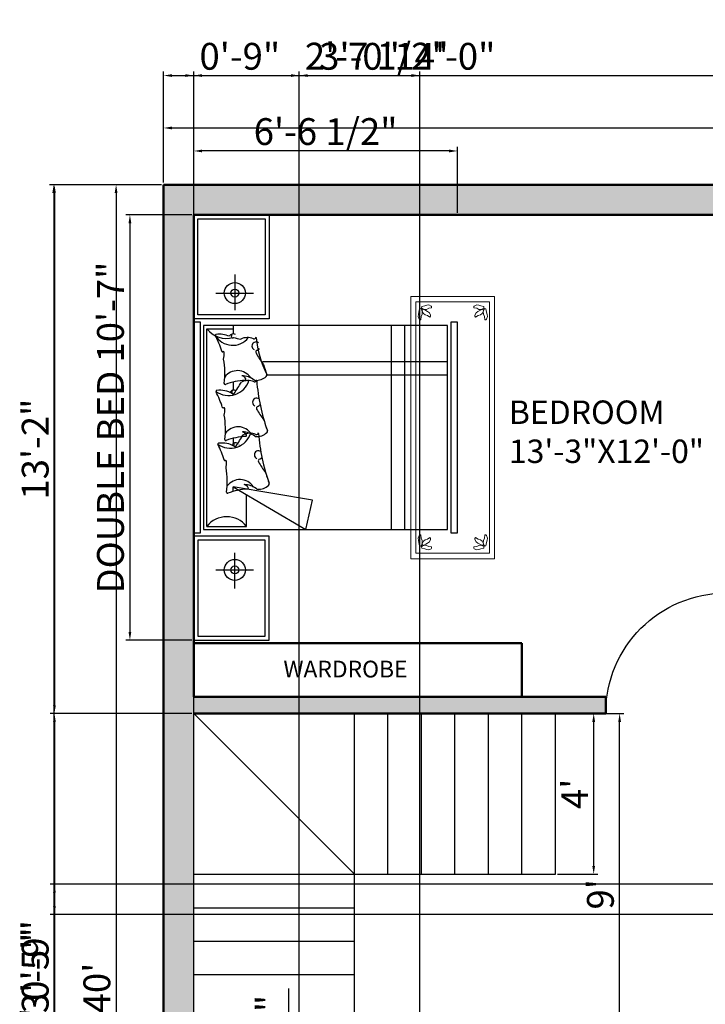
# Model space of a CAD drawing. Units: inches. Extents: x 1770 to 3141, y 984 to 1614.
# Tile 3 of 12: x 1770 to 1974, y 1320 to 1614. Entities that reach past the tile are written whole.
import ezdxf

# ---------------------------------------------------------------- set-up
doc = ezdxf.new("R2010")
doc.units = ezdxf.units.IN
for name, color, linetype, lineweight in [('A-ANNO-DIMS', 2, 'Continuous', 18), ('A-AREA-IDEN', 3, 'Continuous', 18), ('A-DOOR', 4, 'Continuous', 25), ('A-FLOR-STRS', 7, 'Continuous', 25), ('A-FURN', 8, 'Continuous', 18), ('A-WALL', 7, 'Continuous', 50), ('A-WALL-PATT', 8, 'Continuous', 13)]:
    doc.layers.add(name, color=color, linetype=linetype, lineweight=lineweight)
for name, color, linetype in [('FUR', 42, 'Continuous'), ('HA', 9, 'Continuous'), ('HID', 11, 'Continuous'), ('SAN', 5, 'Continuous')]:
    doc.layers.add(name, color=color, linetype=linetype)
doc.styles.get("Standard").update_dxf_attribs({"font": 'arial.ttf'})
doc.dimstyles.new('ISO-25', dxfattribs={"dimtxt": 8, "dimasz": 2.5, "dimexe": 1.25, "dimexo": 0.625, "dimtad": 1, "dimdec": 1, "dimlunit": 3, "dimtxsty": 'Standard', "dimcen": 2.5, "dimclrt": 1, "dimadec": 0, "dimazin": 0, "dimtfac": 1, "dimtdec": 1, "dimtmove": 0, "dimatfit": 3, "dimfxl": 1, "dimarcsym": 0})

# ---------------------------------------------------------------- blocks, each defined once
blk = doc.blocks.new("D1 3'")
for p, q in [((0, 36), (0, 0)), ((1, 36), (1, 0)), ((0, 0), (1, 0))]:
    blk.add_line(p, q)
blk.add_arc((0, 0), 36, 0, 90)
blk = doc.blocks.new('*D17')
at = {"layer": 'A-ANNO-DIMS', "color": 0, "lineweight": -2, "transparency": 16777216}
for p, q in [((1812.73, 1565.8), (1812.73, 1583.37)), ((2412.73, 1565.8), (2412.73, 1583.37)), ((1815.23, 1582.12), (2410.23, 1582.12))]:
    blk.add_line(p, q, dxfattribs=at)
at = {"layer": 'A-ANNO-DIMS', "color": 0, "transparency": 16777216}
for points in [[(1815.23, 1582.54), (1815.23, 1581.7), (1812.73, 1582.12)], [(2410.23, 1582.54), (2410.23, 1581.7), (2412.73, 1582.12)]]:
    blk.add_solid(points, dxfattribs=at)
at = {"layer": 'Defpoints', "color": 0, "transparency": 16777216}
for p in [(2412.73, 1582.12), (1812.73, 1565.18), (2412.73, 1565.18)]:
    blk.add_point(p, dxfattribs=at)
at = {"layer": 'A-ANNO-DIMS', "color": 0, "transparency": 16777216, "insert": (2112.73, 1586.83), "char_height": 8, "attachment_point": 5}
blk.add_mtext("50'", dxfattribs=at)
blk = doc.blocks.new('*D18')
at = {"layer": 'A-ANNO-DIMS', "color": 0, "lineweight": -2, "transparency": 16777216}
for p, q in [((1812.11, 1565.18), (1797.29, 1565.18)), ((1798.54, 1562.68), (1798.54, 1087.68)), ((1812.11, 1085.18), (1797.29, 1085.18))]:
    blk.add_line(p, q, dxfattribs=at)
at = {"layer": 'A-ANNO-DIMS', "color": 0, "transparency": 16777216}
for points in [[(1798.12, 1562.68), (1798.96, 1562.68), (1798.54, 1565.18)], [(1798.12, 1087.68), (1798.96, 1087.68), (1798.54, 1085.18)]]:
    blk.add_solid(points, dxfattribs=at)
at = {"layer": 'Defpoints', "color": 0, "transparency": 16777216}
for p in [(1812.73, 1565.18), (1798.54, 1085.18), (1812.73, 1085.18)]:
    blk.add_point(p, dxfattribs=at)
at = {"layer": 'A-ANNO-DIMS', "color": 0, "transparency": 16777216, "insert": (1793.83, 1325.18), "char_height": 8, "attachment_point": 5, "rotation": 90}
blk.add_mtext("40'", dxfattribs=at)
blk = doc.blocks.new('carpet-7')
at = {"color": 0, "linetype": 'ByBlock'}
for p, q in [((-1.0224, 0), (0, 0)), ((0, 0), (0, -0.54)), ((-1.694, -0.54), (-1.694, 0)), ((-1.694, 0), (-1.0224, 0)), ((-1.658, -0.5076), (-1.658, -0.0324)), ((-1.658, -0.0324), (-0.036, -0.0324)), ((-1.6112, -0.0562), (-1.6124, -0.0637)), ((-1.5896, -0.0518), (-1.6112, -0.0562)), ((-1.5752, -0.0486), (-1.5896, -0.0518)), ((-1.5608, -0.0464), (-1.5752, -0.0486)), ((-1.544, -0.0529), (-1.5608, -0.0464)), ((-1.5404, -0.0562), (-1.544, -0.0529)), ((-1.5404, -0.0637), (-1.5404, -0.0562)), ((-0.1512, -0.0562), (-0.1476, -0.0529)), ((-0.1512, -0.0637), (-0.1512, -0.0562)), ((-0.1476, -0.0529), (-0.1308, -0.0464)), ((-0.1308, -0.0464), (-0.1164, -0.0486)), ((-0.1164, -0.0486), (-0.102, -0.0518)), ((-0.102, -0.0518), (-0.0804, -0.0562)), ((-0.0804, -0.0562), (-0.0792, -0.0637)), ((-0.036, -0.0324), (-0.036, -0.5076)), ((-1.6364, -0.1156), (-1.634, -0.1026)), ((-1.6292, -0.1307), (-1.6364, -0.1156)), ((-1.634, -0.1026), (-1.6304, -0.0896)), ((-1.6304, -0.0896), (-1.6256, -0.0702)), ((-1.6256, -0.0702), (-1.6172, -0.0691)), ((-1.6172, -0.0691), (-1.6124, -0.0724)), ((-1.6148, -0.1156), (-1.6172, -0.1339)), ((-1.6076, -0.1015), (-1.6148, -0.1156)), ((-1.6124, -0.0637), (-1.6088, -0.068)), ((-1.6124, -0.0724), (-1.6064, -0.0886)), ((-1.6088, -0.068), (-1.5908, -0.0734)), ((-1.6088, -0.0788), (-1.6028, -0.0724)), ((-1.5992, -0.0961), (-1.6088, -0.0788)), ((-1.6064, -0.0886), (-1.6076, -0.1015)), ((-1.6028, -0.0724), (-1.5968, -0.0724)), ((-1.5932, -0.108), (-1.5992, -0.0961)), ((-1.5968, -0.0724), (-1.5812, -0.081)), ((-1.5848, -0.1199), (-1.5932, -0.108)), ((-1.5908, -0.0734), (-1.5764, -0.0724)), ((-1.5692, -0.1274), (-1.5848, -0.1199)), ((-1.5812, -0.081), (-1.5728, -0.0918)), ((-1.5764, -0.0724), (-1.5608, -0.0659)), ((-1.5728, -0.0918), (-1.568, -0.1069)), ((-1.568, -0.1069), (-1.5572, -0.1231)), ((-1.5572, -0.1231), (-1.5632, -0.1274)), ((-1.5608, -0.0659), (-1.5404, -0.0637)), ((-0.1308, -0.0659), (-0.1512, -0.0637)), ((-0.1236, -0.1069), (-0.1344, -0.1231)), ((-0.1344, -0.1231), (-0.1284, -0.1274)), ((-0.1152, -0.0724), (-0.1308, -0.0659)), ((-0.1188, -0.0918), (-0.1236, -0.1069)), ((-0.1224, -0.1274), (-0.1068, -0.1199)), ((-0.1104, -0.081), (-0.1188, -0.0918)), ((-0.1008, -0.0734), (-0.1152, -0.0724)), ((-0.0948, -0.0724), (-0.1104, -0.081)), ((-0.1068, -0.1199), (-0.0984, -0.108)), ((-0.0828, -0.068), (-0.1008, -0.0734)), ((-0.0984, -0.108), (-0.0924, -0.0961)), ((-0.0888, -0.0724), (-0.0948, -0.0724)), ((-0.0924, -0.0961), (-0.0828, -0.0788)), ((-0.0828, -0.0788), (-0.0888, -0.0724)), ((-0.0792, -0.0724), (-0.0852, -0.0886)), ((-0.0852, -0.0886), (-0.084, -0.1015)), ((-0.084, -0.1015), (-0.0768, -0.1156)), ((-0.0792, -0.0637), (-0.0828, -0.068)), ((-0.0744, -0.0691), (-0.0792, -0.0724)), ((-0.0768, -0.1156), (-0.0744, -0.1339)), ((-0.066, -0.0702), (-0.0744, -0.0691)), ((-0.0612, -0.0896), (-0.066, -0.0702)), ((-0.0624, -0.1307), (-0.0552, -0.1156)), ((-0.0576, -0.1026), (-0.0612, -0.0896)), ((-0.0552, -0.1156), (-0.0576, -0.1026)), ((-1.6256, -0.1339), (-1.6292, -0.1307)), ((-1.6172, -0.1339), (-1.6256, -0.1339)), ((-1.5632, -0.1274), (-1.5692, -0.1274)), ((-0.1284, -0.1274), (-0.1224, -0.1274)), ((-0.0744, -0.1339), (-0.066, -0.1339)), ((-0.066, -0.1339), (-0.0624, -0.1307)), ((-1.6292, -0.4093), (-1.6364, -0.4244)), ((-1.6364, -0.4244), (-1.634, -0.4374)), ((-1.634, -0.4374), (-1.6304, -0.4504)), ((-1.6256, -0.4061), (-1.6292, -0.4093)), ((-1.6172, -0.4061), (-1.6256, -0.4061)), ((-1.6148, -0.4244), (-1.6172, -0.4061)), ((-1.6076, -0.4385), (-1.6148, -0.4244)), ((-1.5992, -0.4439), (-1.6088, -0.4612)), ((-1.6064, -0.4514), (-1.6076, -0.4385)), ((-1.5932, -0.432), (-1.5992, -0.4439)), ((-1.5848, -0.4201), (-1.5932, -0.432)), ((-1.5692, -0.4126), (-1.5848, -0.4201)), ((-1.5728, -0.4482), (-1.568, -0.4331)), ((-1.5632, -0.4126), (-1.5692, -0.4126)), ((-1.568, -0.4331), (-1.5572, -0.4169)), ((-1.5572, -0.4169), (-1.5632, -0.4126)), ((-0.1344, -0.4169), (-0.1284, -0.4126)), ((-0.1236, -0.4331), (-0.1344, -0.4169)), ((-0.1284, -0.4126), (-0.1224, -0.4126)), ((-0.1188, -0.4482), (-0.1236, -0.4331)), ((-0.1224, -0.4126), (-0.1068, -0.4201)), ((-0.1068, -0.4201), (-0.0984, -0.432)), ((-0.0984, -0.432), (-0.0924, -0.4439)), ((-0.0924, -0.4439), (-0.0828, -0.4612)), ((-0.0852, -0.4514), (-0.084, -0.4385)), ((-0.084, -0.4385), (-0.0768, -0.4244)), ((-0.0768, -0.4244), (-0.0744, -0.4061)), ((-0.0744, -0.4061), (-0.066, -0.4061)), ((-0.066, -0.4061), (-0.0624, -0.4093)), ((-0.0624, -0.4093), (-0.0552, -0.4244)), ((-0.0576, -0.4374), (-0.0612, -0.4504)), ((-0.0552, -0.4244), (-0.0576, -0.4374)), ((-1.658, -0.5076), (-0.036, -0.5076)), ((-1.6304, -0.4504), (-1.6256, -0.4698)), ((-1.6256, -0.4698), (-1.6172, -0.4709)), ((-1.6172, -0.4709), (-1.6124, -0.4676)), ((-1.6124, -0.4676), (-1.6064, -0.4514)), ((-1.6124, -0.4763), (-1.6088, -0.472)), ((-1.6112, -0.4838), (-1.6124, -0.4763)), ((-1.5896, -0.4882), (-1.6112, -0.4838)), ((-1.6088, -0.4612), (-1.6028, -0.4676)), ((-1.6088, -0.472), (-1.5908, -0.4666)), ((-1.6028, -0.4676), (-1.5968, -0.4676)), ((-1.5968, -0.4676), (-1.5812, -0.459)), ((-1.5908, -0.4666), (-1.5764, -0.4676)), ((-1.5752, -0.4914), (-1.5896, -0.4882)), ((-1.5812, -0.459), (-1.5728, -0.4482)), ((-1.5764, -0.4676), (-1.5608, -0.4741)), ((-1.5608, -0.4936), (-1.5752, -0.4914)), ((-1.5608, -0.4741), (-1.5404, -0.4763)), ((-1.544, -0.4871), (-1.5608, -0.4936)), ((-1.5404, -0.4838), (-1.544, -0.4871)), ((-1.5404, -0.4763), (-1.5404, -0.4838)), ((-0.1308, -0.4741), (-0.1512, -0.4763)), ((-0.1512, -0.4763), (-0.1512, -0.4838)), ((-0.1512, -0.4838), (-0.1476, -0.4871)), ((-0.1476, -0.4871), (-0.1308, -0.4936)), ((-0.1152, -0.4676), (-0.1308, -0.4741)), ((-0.1308, -0.4936), (-0.1164, -0.4914)), ((-0.1104, -0.459), (-0.1188, -0.4482)), ((-0.1164, -0.4914), (-0.102, -0.4882)), ((-0.1008, -0.4666), (-0.1152, -0.4676)), ((-0.0948, -0.4676), (-0.1104, -0.459)), ((-0.102, -0.4882), (-0.0804, -0.4838)), ((-0.0828, -0.472), (-0.1008, -0.4666)), ((-0.0888, -0.4676), (-0.0948, -0.4676)), ((-0.0828, -0.4612), (-0.0888, -0.4676)), ((-0.0792, -0.4676), (-0.0852, -0.4514)), ((-0.0792, -0.4763), (-0.0828, -0.472)), ((-0.0804, -0.4838), (-0.0792, -0.4763)), ((-0.0744, -0.4709), (-0.0792, -0.4676)), ((-0.066, -0.4698), (-0.0744, -0.4709)), ((-0.0612, -0.4504), (-0.066, -0.4698)), ((0, -0.54), (-1.694, -0.54))]:
    blk.add_line(p, q, dxfattribs=at)
blk = doc.blocks.new('A$C73A16738')
at = {"layer": 'FUR'}
for p, q in [((1.15, 2.3893), (1.1, 2.1643)), ((1.7, 2.0643), (1.15, 2.3893)), ((1.6, 2.3643), (1.6, 2.1234)), ((1.9, 2.3643), (1.6, 2.3643)), ((1.9, 2.3643), (1.9, 0.8643)), ((1.1, 2.1643), (1.7, 2.0643)), ((1.7, 2.099), (1.7, 2.0643)), ((1.7, 1.6955), (1.7, 1.7349)), ((1.7, 1.2682), (1.7, 1.3299)), ((1.7, 0.8393), (1.7, 0.9036)), ((1.9, 0.8643), (1.7, 0.8643))]:
    blk.add_line(p, q, dxfattribs=at)
for points in [[(1.428, 2.4393), (2, 2.4393), (2, 3.2287), (1.428, 3.2287)], [(1.458, 2.4693), (1.97, 2.4693), (1.97, 3.1987), (1.458, 3.1987)], [(0, 2.4143), (0, 0.8143), (0.05, 0.8143), (0.05, 2.4143)], [(1.95, 2.4143), (1.95, 0.8143), (2, 0.8143), (2, 2.4143)], [(0.075, 0.8393), (1.925, 0.8393), (1.925, 2.3893), (0.075, 2.3893)], [(1.428, 0.7893), (2, 0.7893), (2, 0), (1.428, 0)], [(1.458, 0.7593), (1.97, 0.7593), (1.97, 0.03), (1.458, 0.03)]]:
    blk.add_lwpolyline(points, close=True, dxfattribs=at)
for centre, start, end in [((1.75, 2.4806), 217.78263, 322.21737), ((1.75, 0.7481), 37.78263, 105.27469)]:
    blk.add_arc(centre, 0.1898, start, end, dxfattribs=at)
at = {"layer": 'HA'}
for p, q in [((0.4, 2.3893), (0.4, 0.8393)), ((0.5, 2.3893), (0.5, 0.8393)), ((1.4456, 1.2143), (0.075, 1.2143)), ((1.4772, 1.1143), (0.075, 1.1143))]:
    blk.add_line(p, q, dxfattribs=at)
at = {"layer": 'HID'}
for centre, radius, start, end in [((1.5692, 2.5605), 0.4796, 272.73629, 290.95899), ((1.7434, 2.1059), 0.0072, 352.72477, 110.95899), ((2.3483, 2.0286), 0.6026, 172.72477, 190.27016), ((1.4417, 2.0424), 0.0144, 131.66603, 199.44651), ((0.016, 1.539), 1.4976, 4.58522, 19.44651), ((0.016, 1.539), 1.4976, 16.38601, 19.44651), ((1.5102, 1.9654), 0.1174, 87.33771, 131.66603), ((1.515, 2.0683), 0.0144, 51.60711, 87.33771), ((1.6169, 2.1969), 0.1496, 231.60711, 269.78448), ((1.6496, 2.1284), 0.1197, 212.76276, 323.89219), ((1.5925, 2.0742), 0.0072, 92.73629, 208.29854), ((1.628, 2.0933), 0.0475, 208.29854, 255.78909), ((1.4666, 1.9655), 0.0144, 196.38601, 223.79553), ((0.9264, 1.5508), 0.6667, 29.04896, 37.38232), ((1.4966, 1.8675), 0.0144, 282.64257, 29.04896), ((2.0379, 1.8684), 0.2875, 169.41677, 179.30852), ((1.7576, 1.8718), 0.0072, 179.30852, 290.68903), ((1.5097, 1.8233), 0.0319, 112.70152, 147.15561), ((1.5097, 1.8214), 0.0305, 232.35651, 65.77621), ((1.5029, 1.8394), 0.0144, 102.64257, 112.70152), ((1.7627, 1.8583), 0.0072, 16.21957, 110.68903), ((2.3483, 2.0286), 0.6026, 196.21957, 208.21138), ((1.7225, 1.6087), 0.1623, 53.89466, 162.39517), ((2.8537, 0.9606), 1.4182, 145.83293, 150.02451), ((3.1426, 2.3695), 1.6108, 202.70178, 202.72062), ((1.6834, 1.7584), 0.0288, 232.66199, 339.15728), ((1.6862, 1.7531), 0.0072, 38.83153, 145.83293), ((1.788, 1.9236), 0.1919, 239.92106, 277.12402), ((0.088, 1.8308), 1.6108, 356.49824, 357.28883), ((1.8109, 1.7404), 0.0072, 277.12402, 28.21138), ((1.8109, 1.7404), 0.0072, 277.12402, 28.21138), ((1.4554, 1.6425), 0.0144, 131.66603, 199.44651), ((1.5239, 1.5655), 0.1174, 87.33771, 131.66603), ((1.5236, 1.6535), 0.0144, 67.16626, 184.34216), ((1.5745, 1.7743), 0.1167, 247.16626, 295.7613), ((1.5287, 1.6684), 0.0144, 51.60711, 87.33771), ((1.6306, 1.797), 0.1496, 231.60711, 269.78448), ((1.6633, 1.7284), 0.1197, 212.76276, 323.89219), ((1.6062, 1.6743), 0.0072, 92.73629, 208.29854), ((1.6417, 1.6934), 0.0475, 208.29854, 255.78909), ((1.5829, 2.1606), 0.4796, 272.73629, 290.95899), ((1.7571, 1.706), 0.0072, 352.72477, 110.95899), ((2.362, 1.6287), 0.6026, 172.72477, 190.27016), ((0.0297, 1.1391), 1.4976, 4.58522, 19.44651), ((0.0297, 1.1391), 1.4976, 16.38601, 19.44651), ((1.4803, 1.5656), 0.0144, 196.38601, 223.79553), ((0.9401, 1.1509), 0.6667, 29.04896, 37.38232), ((2.0516, 1.4685), 0.2875, 169.41677, 179.30852), ((1.5234, 1.4234), 0.0319, 112.70152, 147.15561), ((1.5234, 1.4215), 0.0305, 232.35651, 65.77621), ((1.5166, 1.4395), 0.0144, 102.64257, 112.70152), ((1.5103, 1.4676), 0.0144, 282.64257, 29.04896), ((1.7713, 1.4719), 0.0072, 179.30852, 290.68903), ((1.7764, 1.4584), 0.0072, 16.21957, 110.68903), ((2.362, 1.6287), 0.6026, 196.21957, 208.21138), ((1.7362, 1.2088), 0.1623, 53.89466, 162.39517), ((2.8674, 0.5607), 1.4182, 145.83293, 150.02451), ((3.1563, 1.9695), 1.6108, 202.70178, 202.72062), ((1.6971, 1.3585), 0.0288, 232.66199, 339.15728), ((1.6999, 1.3531), 0.0072, 38.83153, 145.83293), ((1.8017, 1.5237), 0.1919, 239.92106, 277.12402), ((0.1017, 1.4309), 1.6108, 356.49824, 357.28883), ((1.5877, 1.7344), 0.4796, 272.73629, 290.95899), ((1.7618, 1.2798), 0.0072, 352.72477, 110.95899), ((2.3667, 1.2026), 0.6026, 172.72477, 190.27016), ((1.8246, 1.3404), 0.0072, 277.12402, 28.21138), ((1.8246, 1.3404), 0.0072, 277.12402, 28.21138), ((1.4601, 1.2163), 0.0144, 131.66603, 199.44651), ((0.6883, 0.8412), 0.8439, 6.22401, 26.03262), ((0.0344, 0.713), 1.4976, 16.38601, 19.44651), ((1.5286, 1.1394), 0.1174, 87.33771, 131.66603), ((1.5373, 1.2536), 0.0144, 67.16626, 184.34216), ((1.5334, 1.2423), 0.0144, 51.60711, 87.33771), ((1.6353, 1.3709), 0.1496, 231.60711, 269.78448), ((1.5882, 1.3744), 0.1167, 247.16626, 295.7613), ((1.6681, 1.3023), 0.1197, 212.76276, 323.89219), ((1.6109, 1.2482), 0.0072, 92.73629, 208.29854), ((1.6464, 1.2673), 0.0475, 208.29854, 255.78909), ((1.485, 1.1395), 0.0144, 196.38601, 223.79553), ((0.9449, 0.7248), 0.6667, 29.04896, 37.38232), ((1.5151, 1.0415), 0.0144, 282.64257, 29.04896), ((2.0564, 1.0424), 0.2875, 169.41677, 179.30852), ((1.5281, 0.9972), 0.0319, 112.70152, 147.15561), ((1.5282, 0.9954), 0.0305, 232.35651, 65.77621), ((1.5214, 1.0134), 0.0144, 102.64257, 112.70152), ((1.7054, 0.84), 0.1504, 29.35981, 142.42811), ((1.7761, 1.0457), 0.0072, 179.30852, 290.68903), ((1.7812, 1.0323), 0.0072, 16.21957, 110.68903), ((2.3667, 1.2026), 0.6026, 196.21957, 208.21138), ((1.5421, 0.9274), 0.0144, 67.16626, 184.34216), ((1.5929, 1.0482), 0.1167, 247.16626, 295.7613), ((1.5813, 0.5283), 0.4195, 73.75237, 81.4605), ((3.1611, 1.5434), 1.6108, 202.70178, 202.72062), ((1.7018, 0.9324), 0.0288, 232.66199, 339.15728), ((1.7047, 0.927), 0.0072, 38.83153, 145.83293), ((0.1065, 1.0048), 1.6108, 356.49824, 357.28883), ((1.8064, 1.0976), 0.1919, 246.10926, 277.12402), ((1.8293, 0.9143), 0.0072, 277.12402, 28.21138), ((1.8293, 0.9143), 0.0072, 277.12402, 28.21138)]:
    blk.add_arc(centre, radius, start, end, dxfattribs=at)
at = {"layer": 'SAN'}
for p, q in [((1.6885, 2.8351), (1.6885, 2.5658)), ((1.8316, 2.6947), (1.5465, 2.6947)), ((1.6885, 0.4536), (1.6885, 0.7229)), ((1.8316, 0.594), (1.5465, 0.594))]:
    blk.add_line(p, q, dxfattribs=at)
for centre, radius in [((1.6885, 2.6947), 0.08), ((1.6885, 2.6947), 0.03), ((1.6885, 0.594), 0.08), ((1.6885, 0.594), 0.03)]:
    blk.add_circle(centre, radius, dxfattribs=at)
blk = doc.blocks.new('*D58')
at = {"layer": 'A-ANNO-DIMS', "color": 0, "lineweight": -2, "transparency": 16777216}
for p, q in [((1930.36, 1407.18), (1942.4, 1407.18)), ((1941.15, 1361.68), (1941.15, 1404.68)), ((1930.36, 1359.18), (1942.4, 1359.18))]:
    blk.add_line(p, q, dxfattribs=at)
at = {"layer": 'A-ANNO-DIMS', "color": 0, "transparency": 16777216}
for points in [[(1940.74, 1404.68), (1941.57, 1404.68), (1941.15, 1407.18)], [(1940.74, 1361.68), (1941.57, 1361.68), (1941.15, 1359.18)]]:
    blk.add_solid(points, dxfattribs=at)
at = {"layer": 'Defpoints', "color": 0, "transparency": 16777216}
for p in [(1929.73, 1407.18), (1941.15, 1407.18), (1929.73, 1359.18)]:
    blk.add_point(p, dxfattribs=at)
at = {"layer": 'A-ANNO-DIMS', "color": 0, "transparency": 16777216, "insert": (1936.53, 1383.18), "char_height": 8, "attachment_point": 5, "rotation": 90}
blk.add_mtext("4'", dxfattribs=at)
blk = doc.blocks.new('*D61')
at = {"layer": 'A-ANNO-DIMS', "color": 0, "lineweight": -2, "transparency": 16777216}
for p, q in [((1910.36, 1407.18), (1950.15, 1407.18)), ((1948.9, 1301.68), (1948.9, 1404.68)), ((1910.36, 1299.18), (1950.15, 1299.18))]:
    blk.add_line(p, q, dxfattribs=at)
at = {"layer": 'A-ANNO-DIMS', "color": 0, "transparency": 16777216}
for points in [[(1948.49, 1404.68), (1949.32, 1404.68), (1948.9, 1407.18)], [(1948.49, 1301.68), (1949.32, 1301.68), (1948.9, 1299.18)]]:
    blk.add_solid(points, dxfattribs=at)
at = {"layer": 'Defpoints', "color": 0, "transparency": 16777216}
for p in [(1909.73, 1407.18), (1948.9, 1407.18), (1909.73, 1299.18)]:
    blk.add_point(p, dxfattribs=at)
at = {"layer": 'A-ANNO-DIMS', "color": 0, "transparency": 16777216, "insert": (1944.19, 1353.18), "char_height": 8, "attachment_point": 5, "rotation": 90}
blk.add_mtext("9'", dxfattribs=at)
blk = doc.blocks.new('*D65')
at = {"layer": 'A-ANNO-DIMS', "color": 0, "lineweight": -2, "transparency": 16777216}
for p, q in [((1812.11, 1565.18), (1778.67, 1565.18)), ((1779.92, 1562.68), (1779.92, 1045.68)), ((1812.11, 1043.18), (1778.67, 1043.18))]:
    blk.add_line(p, q, dxfattribs=at)
at = {"layer": 'A-ANNO-DIMS', "color": 0, "transparency": 16777216}
for points in [[(1779.51, 1562.68), (1780.34, 1562.68), (1779.92, 1565.18)], [(1779.51, 1045.68), (1780.34, 1045.68), (1779.92, 1043.18)]]:
    blk.add_solid(points, dxfattribs=at)
at = {"layer": 'Defpoints', "color": 0, "transparency": 16777216}
for p in [(1812.73, 1565.18), (1779.92, 1043.18), (1812.73, 1043.18)]:
    blk.add_point(p, dxfattribs=at)
at = {"layer": 'A-ANNO-DIMS', "color": 0, "transparency": 16777216, "insert": (1775.21, 1304.18), "char_height": 8, "attachment_point": 5, "rotation": 90}
blk.add_mtext('43\'-6"', dxfattribs=at)
blk = doc.blocks.new('*D84')
at = {"layer": 'A-ANNO-DIMS', "color": 0, "lineweight": -2, "transparency": 16777216}
for p, q in [((1850.13, 1222.14), (1850.13, 1325.01)), ((1845.36, 1222.14), (1851.38, 1222.14)), ((1850.13, 1188.64), (1850.13, 1219.64)), ((1845.36, 1186.14), (1851.38, 1186.14))]:
    blk.add_line(p, q, dxfattribs=at)
at = {"layer": 'A-ANNO-DIMS', "color": 0, "transparency": 16777216}
for points in [[(1849.72, 1219.64), (1850.55, 1219.64), (1850.13, 1222.14)], [(1849.72, 1188.64), (1850.55, 1188.64), (1850.13, 1186.14)]]:
    blk.add_solid(points, dxfattribs=at)
at = {"layer": 'Defpoints', "color": 0, "transparency": 16777216}
for p in [(1844.73, 1222.14), (1850.13, 1222.14), (1844.73, 1186.14)]:
    blk.add_point(p, dxfattribs=at)
at = {"layer": 'A-ANNO-DIMS', "color": 1, "transparency": 16777216, "insert": (1845.37, 1274.82), "char_height": 8, "attachment_point": 5, "rotation": 90}
blk.add_mtext('DOUBLE SINK 3\'-0"', dxfattribs=at)
blk = doc.blocks.new('*D94')
at = {"layer": 'A-ANNO-DIMS', "color": 0, "lineweight": -2, "transparency": 16777216}
for p, q in [((1821.11, 1556.18), (1801.42, 1556.18)), ((1802.67, 1553.68), (1802.67, 1431.57)), ((1821.11, 1429.07), (1801.42, 1429.07))]:
    blk.add_line(p, q, dxfattribs=at)
at = {"layer": 'A-ANNO-DIMS', "color": 0, "transparency": 16777216}
for points in [[(1802.25, 1553.68), (1803.08, 1553.68), (1802.67, 1556.18)], [(1802.25, 1431.57), (1803.08, 1431.57), (1802.67, 1429.07)]]:
    blk.add_solid(points, dxfattribs=at)
at = {"layer": 'Defpoints', "color": 0, "transparency": 16777216}
for p in [(1821.73, 1556.18), (1802.67, 1429.07), (1821.73, 1429.07)]:
    blk.add_point(p, dxfattribs=at)
at = {"layer": 'A-ANNO-DIMS', "color": 1, "transparency": 16777216, "insert": (1797.9, 1492.62), "char_height": 8, "attachment_point": 5, "rotation": 90}
blk.add_mtext('DOUBLE BED 10\'-7"', dxfattribs=at)
blk = doc.blocks.new('*D95')
at = {"layer": 'A-ANNO-DIMS', "color": 0, "lineweight": -2, "transparency": 16777216}
for p, q in [((1821.73, 1556.8), (1821.73, 1576.5)), ((1897.97, 1575.25), (1824.23, 1575.25)), ((1900.47, 1556.8), (1900.47, 1576.5))]:
    blk.add_line(p, q, dxfattribs=at)
at = {"layer": 'A-ANNO-DIMS', "color": 0, "transparency": 16777216}
for points in [[(1824.23, 1575.66), (1824.23, 1574.83), (1821.73, 1575.25)], [(1897.97, 1575.66), (1897.97, 1574.83), (1900.47, 1575.25)]]:
    blk.add_solid(points, dxfattribs=at)
at = {"layer": 'Defpoints', "color": 0, "transparency": 16777216}
for p in [(1821.73, 1575.25), (1821.73, 1556.18), (1900.47, 1556.18)]:
    blk.add_point(p, dxfattribs=at)
at = {"layer": 'A-ANNO-DIMS', "color": 1, "transparency": 16777216, "insert": (1861.1, 1580.01), "char_height": 8, "attachment_point": 5}
blk.add_mtext('6\'-6 1/2"', dxfattribs=at)
blk = doc.blocks.new('*D100')
at = {"layer": 'A-ANNO-DIMS', "color": 0, "lineweight": -2, "transparency": 16777216}
for p, q in [((1812.73, 1565.8), (1812.73, 1599.03)), ((1815.23, 1597.78), (1978.23, 1597.78)), ((1980.73, 1556.8), (1980.73, 1599.03))]:
    blk.add_line(p, q, dxfattribs=at)
at = {"layer": 'A-ANNO-DIMS', "color": 0, "transparency": 16777216}
for points in [[(1815.23, 1598.2), (1815.23, 1597.36), (1812.73, 1597.78)], [(1978.23, 1598.2), (1978.23, 1597.36), (1980.73, 1597.78)]]:
    blk.add_solid(points, dxfattribs=at)
at = {"layer": 'Defpoints', "color": 0, "transparency": 16777216}
for p in [(1980.73, 1597.78), (1812.73, 1565.18), (1980.73, 1556.18)]:
    blk.add_point(p, dxfattribs=at)
at = {"layer": 'A-ANNO-DIMS', "color": 1, "transparency": 16777216, "insert": (1896.73, 1602.49), "char_height": 8, "attachment_point": 5}
blk.add_mtext('14\'-0"', dxfattribs=at)
blk = doc.blocks.new('*D105')
at = {"layer": 'A-ANNO-DIMS', "color": 0, "lineweight": -2, "transparency": 16777216}
for p, q in [((1812.73, 1565.8), (1812.73, 1599.03)), ((1815.23, 1597.78), (1819.23, 1597.78)), ((1821.73, 1556.8), (1821.73, 1599.03)), ((1821.73, 1597.78), (1846.75, 1597.78))]:
    blk.add_line(p, q, dxfattribs=at)
at = {"layer": 'A-ANNO-DIMS', "color": 0, "transparency": 16777216}
for points in [[(1815.23, 1598.2), (1815.23, 1597.36), (1812.73, 1597.78)], [(1819.23, 1598.2), (1819.23, 1597.36), (1821.73, 1597.78)]]:
    blk.add_solid(points, dxfattribs=at)
at = {"layer": 'Defpoints', "color": 0, "transparency": 16777216}
for p in [(1821.73, 1597.78), (1812.73, 1565.18), (1821.73, 1556.18)]:
    blk.add_point(p, dxfattribs=at)
at = {"layer": 'A-ANNO-DIMS', "color": 1, "transparency": 16777216, "insert": (1835.49, 1602.49), "char_height": 8, "attachment_point": 5}
blk.add_mtext('0\'-9"', dxfattribs=at)
blk = doc.blocks.new('*D107')
at = {"layer": 'A-ANNO-DIMS', "color": 0, "lineweight": -2, "transparency": 16777216}
for p, q in [((1812.11, 1565.18), (1778.88, 1565.18)), ((1780.13, 1562.68), (1780.13, 1409.68)), ((1821.11, 1407.18), (1778.88, 1407.18))]:
    blk.add_line(p, q, dxfattribs=at)
at = {"layer": 'A-ANNO-DIMS', "color": 0, "transparency": 16777216}
for points in [[(1779.72, 1562.68), (1780.55, 1562.68), (1780.13, 1565.18)], [(1779.72, 1409.68), (1780.55, 1409.68), (1780.13, 1407.18)]]:
    blk.add_solid(points, dxfattribs=at)
at = {"layer": 'Defpoints', "color": 0, "transparency": 16777216}
for p in [(1812.73, 1565.18), (1780.13, 1407.18), (1821.73, 1407.18)]:
    blk.add_point(p, dxfattribs=at)
at = {"layer": 'A-ANNO-DIMS', "color": 1, "transparency": 16777216, "insert": (1775.42, 1486.18), "char_height": 8, "attachment_point": 5, "rotation": 90}
blk.add_mtext('13\'-2"', dxfattribs=at)
blk = doc.blocks.new('*D108')
at = {"layer": 'A-ANNO-DIMS', "color": 0, "lineweight": -2, "transparency": 16777216}
for p, q in [((1821.11, 1407.18), (1778.88, 1407.18)), ((1780.13, 1404.68), (1780.13, 1248.68)), ((1821.11, 1246.18), (1778.88, 1246.18))]:
    blk.add_line(p, q, dxfattribs=at)
at = {"layer": 'A-ANNO-DIMS', "color": 0, "transparency": 16777216}
for points in [[(1779.72, 1404.68), (1780.55, 1404.68), (1780.13, 1407.18)], [(1779.72, 1248.68), (1780.55, 1248.68), (1780.13, 1246.18)]]:
    blk.add_solid(points, dxfattribs=at)
at = {"layer": 'Defpoints', "color": 0, "transparency": 16777216}
for p in [(1821.73, 1407.18), (1780.13, 1246.18), (1821.73, 1246.18)]:
    blk.add_point(p, dxfattribs=at)
at = {"layer": 'A-ANNO-DIMS', "color": 1, "transparency": 16777216, "insert": (1775.42, 1326.68), "char_height": 8, "attachment_point": 5, "rotation": 90}
blk.add_mtext('13\'-5"', dxfattribs=at)
blk = doc.blocks.new('*D114')
at = {"layer": 'A-ANNO-DIMS', "color": 0, "lineweight": -2, "transparency": 16777216}
for p, q in [((1821.73, 1094.8), (1821.73, 1599.03)), ((1824.23, 1597.78), (1850.73, 1597.78)), ((1853.23, 1094.8), (1853.23, 1599.03)), ((1853.23, 1597.78), (1897.03, 1597.78))]:
    blk.add_line(p, q, dxfattribs=at)
at = {"layer": 'A-ANNO-DIMS', "color": 0, "transparency": 16777216}
for points in [[(1824.23, 1598.2), (1824.23, 1597.36), (1821.73, 1597.78)], [(1850.73, 1598.2), (1850.73, 1597.36), (1853.23, 1597.78)]]:
    blk.add_solid(points, dxfattribs=at)
at = {"layer": 'Defpoints', "color": 0, "transparency": 16777216}
for p in [(1853.23, 1597.78), (1821.73, 1094.18), (1853.23, 1094.18)]:
    blk.add_point(p, dxfattribs=at)
at = {"layer": 'A-ANNO-DIMS', "color": 1, "transparency": 16777216, "insert": (1876.38, 1602.54), "char_height": 8, "attachment_point": 5}
blk.add_mtext('2\'-7 1/2"', dxfattribs=at)
blk = doc.blocks.new('*D115')
at = {"layer": 'A-ANNO-DIMS', "color": 0, "lineweight": -2, "transparency": 16777216}
for p, q in [((1853.23, 1094.8), (1853.23, 1599.03)), ((1855.73, 1597.78), (1886.73, 1597.78)), ((1889.23, 1094.8), (1889.23, 1599.03))]:
    blk.add_line(p, q, dxfattribs=at)
at = {"layer": 'A-ANNO-DIMS', "color": 0, "transparency": 16777216}
for points in [[(1855.73, 1598.2), (1855.73, 1597.36), (1853.23, 1597.78)], [(1886.73, 1598.2), (1886.73, 1597.36), (1889.23, 1597.78)]]:
    blk.add_solid(points, dxfattribs=at)
at = {"layer": 'Defpoints', "color": 0, "transparency": 16777216}
for p in [(1889.23, 1597.78), (1853.23, 1094.18), (1889.23, 1094.18)]:
    blk.add_point(p, dxfattribs=at)
at = {"layer": 'A-ANNO-DIMS', "color": 1, "transparency": 16777216, "insert": (1871.23, 1602.49), "char_height": 8, "attachment_point": 5}
blk.add_mtext('3\'-0"', dxfattribs=at)
blk = doc.blocks.new('*D120')
at = {"layer": 'A-ANNO-DIMS', "color": 0, "lineweight": -2, "transparency": 16777216}
for p, q in [((2333.11, 1356.18), (1778.88, 1356.18)), ((1780.13, 1353.68), (1780.13, 1349.68)), ((2333.11, 1347.18), (1778.88, 1347.18)), ((1780.13, 1347.18), (1780.13, 1322.16))]:
    blk.add_line(p, q, dxfattribs=at)
at = {"layer": 'A-ANNO-DIMS', "color": 0, "transparency": 16777216}
for points in [[(1779.72, 1353.68), (1780.55, 1353.68), (1780.13, 1356.18)], [(1779.72, 1349.68), (1780.55, 1349.68), (1780.13, 1347.18)]]:
    blk.add_solid(points, dxfattribs=at)
at = {"layer": 'Defpoints', "color": 0, "transparency": 16777216}
for p in [(2333.73, 1356.18), (1780.13, 1347.18), (2333.73, 1347.18)]:
    blk.add_point(p, dxfattribs=at)
at = {"layer": 'A-ANNO-DIMS', "color": 1, "transparency": 16777216, "insert": (1775.42, 1333.42), "char_height": 8, "attachment_point": 5, "rotation": 90}
blk.add_mtext('0\'-9"', dxfattribs=at)

msp = doc.modelspace()

# ---------------------------------------------------------------- hatches: boundary and pattern name
at = {"layer": 'A-WALL-PATT'}
h = msp.add_hatch(color=256, dxfattribs=at)
h.dxf.hatch_style = 1
h.paths.add_polyline_path([(1821.73, 1556.18), (1844.25, 1556.18), (2086.73, 1556.18), (2086.73, 1443.18), (2091.73, 1443.18), (2091.73, 1556.18), (2239.73, 1556.18), (2239.73, 1565.18), (1812.73, 1565.18), (1812.73, 1100.18), (1821.73, 1100.18), (1821.73, 1246.18), (1913.73, 1246.18), (1913.73, 1251.18), (1821.73, 1251.18), (1821.73, 1407.18), (1944.73, 1407.18), (1944.73, 1412.18), (1821.73, 1412.18)])
h.paths.add_polyline_path([(1985.73, 1515.18), (1997.73, 1515.18), (1997.73, 1520.18), (1980.73, 1520.18), (1980.73, 1478.18), (1985.73, 1478.18)], flags=16)
h.paths.add_polyline_path([(2038.73, 1520.18), (2021.73, 1520.18), (2021.73, 1515.18), (2033.73, 1515.18), (2033.73, 1412.18), (1985.73, 1412.18), (1985.73, 1448.18), (1980.73, 1448.18), (1980.73, 1407.18), (2038.73, 1407.18), (2038.73, 1443.18), (2056.73, 1443.18), (2056.73, 1448.18), (2038.73, 1448.18)], flags=17)
h.paths.add_polyline_path([(1853.23, 1094.18), (1821.73, 1094.18), (1821.73, 1085.18), (1853.23, 1085.18)])
h.paths.add_polyline_path([(2001.73, 1094.18), (1966.73, 1094.18), (1966.73, 1124.18), (1961.73, 1124.18), (1961.73, 1094.18), (1889.23, 1094.18), (1889.23, 1085.18), (2001.73, 1085.18)])
h.paths.add_polyline_path([(2020.69, 1094.18), (2010.73, 1094.18), (2010.73, 1085.18), (2020.69, 1085.18)])
h.paths.add_polyline_path([(2116.73, 1094.18), (2080.69, 1094.18), (2080.69, 1085.18), (2116.73, 1085.18)])
h.paths.add_polyline_path([(2125.73, 1184.68), (2116.73, 1184.68), (2116.73, 1159.18), (2056.73, 1159.18), (2056.73, 1246.18), (2086.73, 1246.18), (2086.73, 1251.18), (2001.73, 1251.18), (2001.73, 1246.18), (2051.73, 1246.18), (2051.73, 1159.18), (1966.73, 1159.18), (1966.73, 1246.18), (1971.73, 1246.18), (1971.73, 1251.18), (1961.73, 1251.18), (1961.73, 1154.18), (1991.73, 1154.18), (2125.73, 1154.18)], flags=17)
h.paths.add_polyline_path([(2125.73, 1256.18), (2116.73, 1256.18), (2116.73, 1220.68), (2125.73, 1220.68)], flags=17)
h.paths.add_polyline_path([(2128.73, 1309.18), (2116.73, 1309.18), (2116.73, 1292.18), (2125.73, 1292.18), (2125.73, 1300.18), (2128.73, 1300.18)], flags=17)
h.paths.add_polyline_path([(2239.73, 1309.18), (2217.73, 1309.18), (2217.73, 1300.18), (2239.73, 1300.18)], flags=17)
h.paths.add_polyline_path([(2181.73, 1309.18), (2176.73, 1309.18), (2176.73, 1300.18), (2181.73, 1300.18)], flags=17)

# ---------------------------------------------------------------- linework, layer by layer
at = {"layer": 'A-FLOR-STRS'}
for p, q in [((1821.73, 1251.18), (1821.73, 1407.18)), ((1821.73, 1407.18), (1869.73, 1359.18)), ((1869.73, 1251.18), (1869.73, 1407.18)), ((1879.73, 1359.18), (1879.73, 1407.18)), ((1889.73, 1359.18), (1889.73, 1407.18)), ((1899.73, 1359.18), (1899.73, 1407.18)), ((1909.73, 1359.18), (1909.73, 1407.18)), ((1919.73, 1359.18), (1919.73, 1407.18)), ((1929.73, 1359.18), (1929.73, 1407.18)), ((1821.73, 1359.18), (1929.73, 1359.18)), ((1821.73, 1349.18), (1869.73, 1349.18)), ((1821.73, 1339.18), (1869.73, 1339.18)), ((1821.73, 1329.18), (1869.73, 1329.18))]:
    msp.add_line(p, q, dxfattribs=at)
at = {"layer": 'A-WALL'}
for p, q in [((1812.73, 1565.18), (2412.73, 1565.18)), ((1812.73, 1043.18), (1812.73, 1565.18)), ((1821.73, 1556.18), (2086.73, 1556.18)), ((1821.73, 1412.18), (1821.73, 1556.18)), ((1821.73, 1428.18), (1919.73, 1428.18)), ((1919.73, 1412.18), (1919.73, 1428.18)), ((1821.73, 1412.18), (1944.73, 1412.18)), ((1944.73, 1407.18), (1944.73, 1412.18)), ((1821.73, 1407.18), (1944.73, 1407.18))]:
    msp.add_line(p, q, dxfattribs=at)

# ---------------------------------------------------------------- block references
at = {"layer": 'A-DOOR', "xscale": -1}
msp.add_blockref("D1 3'", (1980.73, 1407.18), dxfattribs=at)
at = {"layer": 'A-FURN'}
for name, p, xscale, yscale, zscale, rotation in [('A$C73A16738', (1900.47, 1556.18), 39.3701, 39.3701, 39.3701, 180), ('carpet-7', (1886.57, 1531.82), 46.2750735389499, 46.2750735389499, 46.2750735389499, 90)]:
    msp.add_blockref(name, p, dxfattribs=dict(at, xscale=xscale, yscale=yscale, zscale=zscale, rotation=rotation))

# ---------------------------------------------------------------- texts
at = {"layer": 'A-AREA-IDEN', "attachment_point": 1}
for s, insert, char_height in [('BEDROOM\\P13\'-3"X12\'-0"', (1915.83, 1500.7), 7), ('WARDROBE', (1848.51, 1422.96), 5)]:
    msp.add_mtext_dynamic_manual_height_columns(s, width=86.9528, gutter_width=12.5, heights=[0], dxfattribs=dict(at, insert=insert, char_height=char_height))

# ---------------------------------------------------------------- dimensions: what is measured, and where the dimension line sits
at = {"layer": 'A-ANNO-DIMS'}
for base, p1, p2, override, picture, middle in [((1853.23, 1597.78), (1821.73, 1094.18), (1853.23, 1094.18), {"dimdec": 1, "dimlfac": 1, "dimrnd": 0, "dimzin": 1, "dimdsep": 46, "dimlunit": 4, "dimfrac": 2}, '*D114', (1876.38, 1602.54)), ((1980.73, 1597.78), (1812.73, 1565.18), (1980.73, 1556.18), {"dimdec": 1, "dimlfac": 1, "dimrnd": 0, "dimzin": 1, "dimdsep": 46, "dimlunit": 4, "dimfrac": 2}, '*D100', (1896.73, 1602.49)), ((1821.73, 1597.78), (1812.73, 1565.18), (1821.73, 1556.18), {"dimdec": 1, "dimlfac": 1, "dimrnd": 0, "dimzin": 1, "dimdsep": 46, "dimlunit": 4, "dimfrac": 2}, '*D105', (1835.49, 1602.49)), ((1889.23, 1597.78), (1853.23, 1094.18), (1889.23, 1094.18), {"dimdec": 1, "dimlfac": 1, "dimrnd": 0, "dimzin": 1, "dimdsep": 46, "dimlunit": 4, "dimfrac": 2}, '*D115', (1871.23, 1602.49)), ((2412.73, 1582.12), (1812.73, 1565.18), (2412.73, 1565.18), {"dimclrd": 0, "dimclre": 0, "dimclrt": 0}, '*D17', (2112.73, 1586.83))]:
    dim = msp.add_linear_dim(base=base, p1=p1, p2=p2, dimstyle='ISO-25', override=override, dxfattribs=at)
    dim.commit()
    dim.dimension.update_dxf_attribs({"geometry": picture, "text_midpoint": middle})
for base, p1, p2, angle, override, picture, middle in [((1821.73, 1575.25), (1900.47, 1556.18), (1821.73, 1556.18), 180, {"dimdec": 1, "dimrnd": 0, "dimzin": 1, "dimlunit": 4, "dimfrac": 2}, '*D95', (1861.1, 1580.01)), ((1779.92, 1043.18), (1812.73, 1565.18), (1812.73, 1043.18), 90, {"dimclrd": 0, "dimclre": 0, "dimclrt": 0}, '*D65', (1775.21, 1304.18)), ((1780.13, 1407.18), (1812.73, 1565.18), (1821.73, 1407.18), 90, {"dimdec": 1, "dimlfac": 1, "dimrnd": 0, "dimzin": 1, "dimdsep": 46, "dimlunit": 4, "dimfrac": 2}, '*D107', (1775.42, 1486.18)), ((1798.54, 1085.18), (1812.73, 1565.18), (1812.73, 1085.18), 90, {"dimclrd": 0, "dimclre": 0, "dimclrt": 0}, '*D18', (1793.83, 1325.18)), ((1780.13, 1246.18), (1821.73, 1407.18), (1821.73, 1246.18), 90, {"dimdec": 1, "dimlfac": 1, "dimrnd": 0, "dimzin": 1, "dimdsep": 46, "dimlunit": 4, "dimfrac": 2}, '*D108', (1775.42, 1326.68)), ((1948.9, 1407.18), (1909.73, 1299.18), (1909.73, 1407.18), 90, {"dimclrd": 0, "dimclre": 0, "dimclrt": 0}, '*D61', (1944.19, 1353.18)), ((1941.15, 1407.18), (1929.73, 1359.18), (1929.73, 1407.18), 90, {"dimclrd": 0, "dimclre": 0, "dimclrt": 0}, '*D58', (1936.53, 1383.18)), ((1780.13, 1347.18), (2333.73, 1356.18), (2333.73, 1347.18), 90, {"dimdec": 1, "dimlfac": 1, "dimrnd": 0, "dimzin": 1, "dimdsep": 46, "dimlunit": 4, "dimfrac": 2}, '*D120', (1775.42, 1333.42))]:
    dim = msp.add_linear_dim(base=base, p1=p1, p2=p2, angle=angle, dimstyle='ISO-25', override=override, dxfattribs=at)
    dim.commit()
    dim.dimension.update_dxf_attribs({"geometry": picture, "text_midpoint": middle})
for base, p1, p2, angle, text, picture, middle in [((1802.67, 1429.07), (1821.73, 1556.18), (1821.73, 1429.07), 270, 'DOUBLE BED <>', '*D94', (1797.9, 1492.62)), ((1850.13, 1222.14), (1844.73, 1186.14), (1844.73, 1222.14), 90, 'DOUBLE SINK <>', '*D84', (1845.37, 1274.82))]:
    dim = msp.add_linear_dim(base=base, p1=p1, p2=p2, angle=angle, text=text, dimstyle='ISO-25', override={"dimdec": 1, "dimrnd": 0, "dimzin": 1, "dimlunit": 4, "dimfrac": 2}, dxfattribs=at)
    dim.commit()
    dim.dimension.update_dxf_attribs({"geometry": picture, "text_midpoint": middle})

doc.saveas('drawing.dxf')
